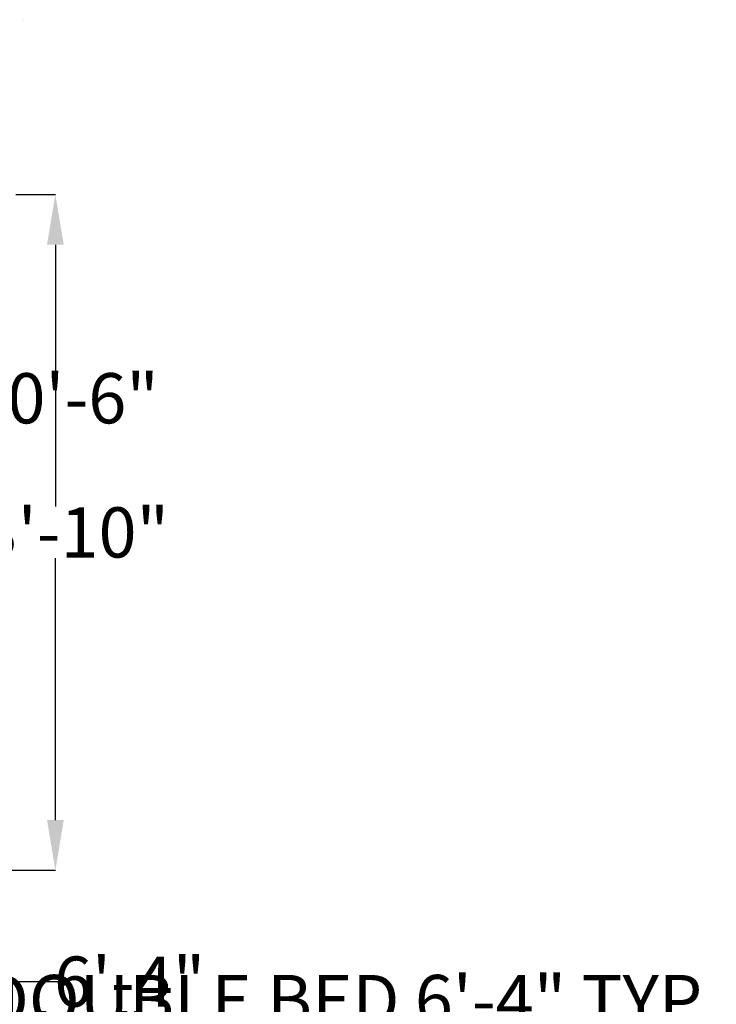
# Model space of a CAD drawing. Units: inches. Extents: x 7323 to 9737, y 2037 to 3322.
# Tile 19 of 19: x 9276 to 9695, y 2709 to 3301. Entities that reach past the tile are written whole.
import ezdxf

# ---------------------------------------------------------------- set-up
doc = ezdxf.new("R2010")
doc.units = ezdxf.units.IN
doc.header["$MEASUREMENT"] = 0
doc.layers.add('A-ANNO-DIMS', color=2, linetype='Continuous', lineweight=18)
doc.layers.add('A-DETL-REFR', color=8, linetype='Continuous', lineweight=13)
doc.styles.get("Standard").update_dxf_attribs({"font": 'arial.ttf'})
doc.dimstyles.get("Standard").update_dxf_attribs({"dimtxt": 30.18, "dimasz": 30.18, "dimexe": 0.18, "dimexo": 0.0625, "dimgap": 0.09, "dimtad": 0, "dimtih": 1, "dimtoh": 1, "dimdec": 0, "dimzin": 0, "dimdsep": 46, "dimlunit": 3, "dimtxsty": 'Standard', "dimcen": 0.09, "dimadec": 0, "dimazin": 0, "dimtfac": 1, "dimtdec": 0, "dimtofl": 0, "dimtmove": 0, "dimatfit": 3, "dimfxl": 1, "dimtolj": 1, "dimtzin": 0, "dimarcsym": 0})

# ---------------------------------------------------------------- blocks, each defined once
blk = doc.blocks.new('*D35')
at = {"layer": 'A-ANNO-DIMS', "color": 0, "lineweight": -2, "transparency": 16777216}
for p, q in [((8977.7, 2688.2), (8947.52, 2688.2)), ((9007.88, 2687.36), (9007.88, 2688.38)), ((9013.95, 2687.36), (9013.95, 2688.38)), ((9044.13, 2688.2), (9074.31, 2688.2))]:
    blk.add_line(p, q, dxfattribs=at)
at = {"layer": 'A-ANNO-DIMS', "color": 0, "transparency": 16777216}
for points in [[(8977.7, 2693.23), (8977.7, 2683.17), (9007.88, 2688.2)], [(9044.13, 2693.23), (9044.13, 2683.17), (9013.95, 2688.2)]]:
    blk.add_solid(points, dxfattribs=at)
at = {"layer": 'Defpoints', "color": 0, "transparency": 16777216}
for p in [(9007.88, 2687.3), (9013.95, 2688.2), (9013.95, 2687.3)]:
    blk.add_point(p, dxfattribs=at)
at = {"layer": 'A-ANNO-DIMS', "color": 0, "transparency": 16777216, "insert": (9263.41, 2688.2), "char_height": 30.18, "attachment_point": 5}
blk.add_mtext('\\A1;COLUMN 0\'-6" TYP.', dxfattribs=at)
blk = doc.blocks.new('*D45')
at = {"layer": 'A-ANNO-DIMS', "color": 0, "lineweight": -2, "transparency": 16777216}
for p, q in [((8725.79, 2664.36), (8695.61, 2664.36)), ((8755.97, 2662.02), (8755.97, 2664.54)), ((8772, 2662.02), (8772, 2664.54)), ((8802.18, 2664.36), (8832.36, 2664.36))]:
    blk.add_line(p, q, dxfattribs=at)
at = {"layer": 'A-ANNO-DIMS', "color": 0, "transparency": 16777216}
for points in [[(8725.79, 2669.39), (8725.79, 2659.33), (8755.97, 2664.36)], [(8802.18, 2669.39), (8802.18, 2659.33), (8772, 2664.36)]]:
    blk.add_solid(points, dxfattribs=at)
at = {"layer": 'Defpoints', "color": 0, "transparency": 16777216}
for p in [(8772, 2664.36), (8755.97, 2661.96), (8772, 2661.96)]:
    blk.add_point(p, dxfattribs=at)
at = {"layer": 'A-ANNO-DIMS', "color": 0, "transparency": 16777216, "insert": (9094.8, 2664.36), "char_height": 30.18, "attachment_point": 5}
blk.add_mtext('\\A1;BEDSIDE TABLE 1\'-4" TYP.', dxfattribs=at)
blk = doc.blocks.new('*D61')
at = {"layer": 'A-ANNO-DIMS', "color": 0, "lineweight": -2, "transparency": 16777216}
for p, q in [((9212.57, 2681.3), (9212.57, 2711.48)), ((9212.57, 2711.48), (9242.75, 2711.48)), ((9201.24, 2681.3), (9212.75, 2681.3)), ((9212.57, 2635.56), (9212.57, 2651.12)), ((9201.24, 2605.38), (9212.75, 2605.38))]:
    blk.add_line(p, q, dxfattribs=at)
at = {"layer": 'A-ANNO-DIMS', "color": 0, "transparency": 16777216}
for points in [[(9207.54, 2651.12), (9217.6, 2651.12), (9212.57, 2681.3)], [(9207.54, 2635.56), (9217.6, 2635.56), (9212.57, 2605.38)]]:
    blk.add_solid(points, dxfattribs=at)
at = {"layer": 'Defpoints', "color": 0, "transparency": 16777216}
for p in [(9201.18, 2681.3), (9212.57, 2681.3), (9201.18, 2605.38)]:
    blk.add_point(p, dxfattribs=at)
at = {"layer": 'A-ANNO-DIMS', "color": 0, "transparency": 16777216, "insert": (9475.82, 2711.48), "char_height": 30.18, "attachment_point": 5}
blk.add_mtext('\\A1;DOUBLE BED 6\'-4" TYP.', dxfattribs=at)
blk = doc.blocks.new('*D93')
at = {"layer": 'A-ANNO-DIMS', "color": 0, "lineweight": -2, "transparency": 16777216}
for p, q in [((9274.01, 3195.71), (9297.98, 3195.71)), ((9297.8, 3165.53), (9297.8, 3008.09)), ((9297.8, 2819.64), (9297.8, 2977.07)), ((9016.27, 2789.46), (9297.98, 2789.46))]:
    blk.add_line(p, q, dxfattribs=at)
at = {"layer": 'A-ANNO-DIMS', "color": 0, "transparency": 16777216}
for points in [[(9292.77, 3165.53), (9302.83, 3165.53), (9297.8, 3195.71)], [(9292.77, 2819.64), (9302.83, 2819.64), (9297.8, 2789.46)]]:
    blk.add_solid(points, dxfattribs=at)
at = {"layer": 'Defpoints', "color": 0, "transparency": 16777216}
for p in [(9273.95, 3195.71), (9297.8, 3195.71), (9016.21, 2789.46)]:
    blk.add_point(p, dxfattribs=at)
at = {"layer": 'A-ANNO-DIMS', "color": 0, "transparency": 16777216, "insert": (9297.8, 2992.58), "char_height": 30.18, "attachment_point": 5}
blk.add_mtext('\\A1;33\'-10"', dxfattribs=at)
blk = doc.blocks.new('*D103')
at = {"layer": 'A-ANNO-DIMS', "color": 0, "lineweight": -2, "transparency": 16777216}
for p, q in [((9244.1, 3043.05), (9244.1, 3073.23)), ((9244.1, 3073.23), (9274.28, 3073.23)), ((9267.89, 3012.87), (9243.92, 3012.87)), ((9267.89, 3006.87), (9243.92, 3006.87)), ((9244.1, 2976.69), (9244.1, 2946.51))]:
    blk.add_line(p, q, dxfattribs=at)
at = {"layer": 'A-ANNO-DIMS', "color": 0, "transparency": 16777216}
for points in [[(9239.07, 3043.05), (9249.13, 3043.05), (9244.1, 3012.87)], [(9239.07, 2976.69), (9249.13, 2976.69), (9244.1, 3006.87)]]:
    blk.add_solid(points, dxfattribs=at)
at = {"layer": 'Defpoints', "color": 0, "transparency": 16777216}
for p in [(9244.1, 3012.87), (9267.95, 3012.87), (9267.95, 3006.87)]:
    blk.add_point(p, dxfattribs=at)
at = {"layer": 'A-ANNO-DIMS', "color": 0, "transparency": 16777216, "insert": (9314.48, 3073.23), "char_height": 30.18, "attachment_point": 5}
blk.add_mtext('\\A1;0\'-6"', dxfattribs=at)
blk = doc.blocks.new('*D123')
at = {"layer": 'A-ANNO-DIMS', "color": 0, "lineweight": -2, "transparency": 16777216}
for p, q in [((9195.95, 2687.36), (9195.95, 2722.73)), ((9226.13, 2722.55), (9241.77, 2722.55)), ((9271.95, 2687.36), (9271.95, 2722.73)), ((9271.95, 2722.55), (9302.13, 2722.55))]:
    blk.add_line(p, q, dxfattribs=at)
at = {"layer": 'A-ANNO-DIMS', "color": 0, "transparency": 16777216}
for points in [[(9226.13, 2727.58), (9226.13, 2717.52), (9195.95, 2722.55)], [(9241.77, 2727.58), (9241.77, 2717.52), (9271.95, 2722.55)]]:
    blk.add_solid(points, dxfattribs=at)
at = {"layer": 'Defpoints', "color": 0, "transparency": 16777216}
for p in [(9271.95, 2722.55), (9195.95, 2687.3), (9271.95, 2687.3)]:
    blk.add_point(p, dxfattribs=at)
at = {"layer": 'A-ANNO-DIMS', "color": 0, "transparency": 16777216, "insert": (9342.41, 2722.55), "char_height": 30.18, "attachment_point": 5}
blk.add_mtext('\\A1;6\'-4"', dxfattribs=at)

msp = doc.modelspace()

# ---------------------------------------------------------------- linework, layer by layer
at = {"layer": 'A-DETL-REFR'}
msp.add_lwpolyline([(9278.77, 3300.81), (9278.77, 3300.81)], close=True, dxfattribs=at)

# ---------------------------------------------------------------- dimensions: what is measured, and where the dimension line sits
at = {"layer": 'A-ANNO-DIMS'}
for base, p1, p2, picture, middle in [((9297.7981, 3195.7082), (9016.212, 2789.4588), (9273.9481, 3195.7082), '*D93', (9297.7981, 2992.5835)), ((9244.1, 3012.87), (9267.95, 3006.87), (9267.95, 3012.87), '*D103', (9314.48, 3073.23))]:
    dim = msp.add_linear_dim(base=base, p1=p1, p2=p2, angle=90, dimstyle='Standard', override={"dimdec": 1, "dimlfac": 1, "dimrnd": 0, "dimzin": 1, "dimdsep": 46, "dimlunit": 4, "dimfrac": 2}, dxfattribs=at)
    dim.commit()
    dim.dimension.update_dxf_attribs({"geometry": picture, "text_midpoint": middle})
dim = msp.add_linear_dim(base=(9212.57, 2681.3), p1=(9201.18, 2605.38), p2=(9201.18, 2681.3), angle=90, text='DOUBLE BED <> TYP.', dimstyle='Standard', override={"dimdec": 1, "dimlfac": 1, "dimrnd": 0, "dimzin": 1, "dimdsep": 46, "dimlunit": 4, "dimfrac": 2}, dxfattribs=at)
dim.commit()
dim.dimension.update_dxf_attribs({"geometry": '*D61', "text_midpoint": (9475.82, 2711.48)})
for base, p1, p2, text, picture, middle in [((8772, 2664.36), (8755.97, 2661.96), (8772, 2661.96), 'BEDSIDE TABLE <> TYP.', '*D45', (9094.8, 2664.36)), ((9013.95, 2688.2), (9007.88, 2687.3), (9013.95, 2687.3), 'COLUMN <> TYP.', '*D35', (9263.41, 2688.2))]:
    dim = msp.add_linear_dim(base=base, p1=p1, p2=p2, text=text, dimstyle='Standard', override={"dimdec": 1, "dimlfac": 1, "dimrnd": 0, "dimzin": 1, "dimdsep": 46, "dimlunit": 4, "dimfrac": 2}, dxfattribs=at)
    dim.commit()
    dim.dimension.update_dxf_attribs({"geometry": picture, "text_midpoint": middle})
dim = msp.add_linear_dim(base=(9271.95, 2722.55), p1=(9195.95, 2687.3), p2=(9271.95, 2687.3), dimstyle='Standard', override={"dimdec": 1, "dimlfac": 1, "dimrnd": 0, "dimzin": 1, "dimdsep": 46, "dimlunit": 4, "dimfrac": 2}, dxfattribs=at)
dim.commit()
dim.dimension.update_dxf_attribs({"geometry": '*D123', "text_midpoint": (9342.41, 2722.55)})

doc.saveas('drawing.dxf')
